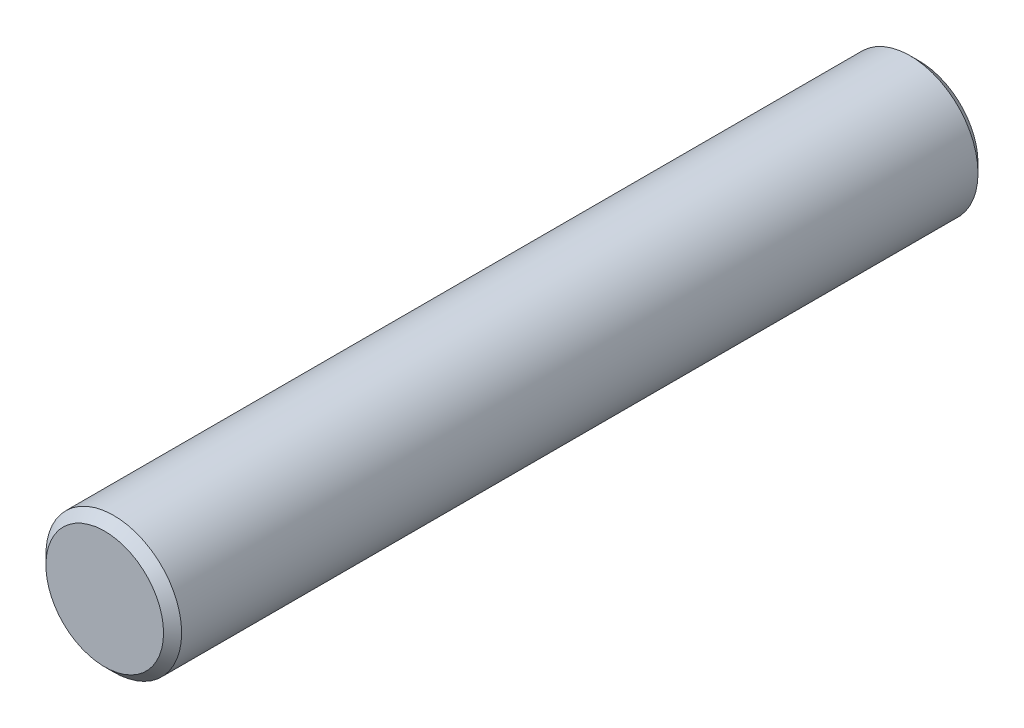
from build123d import *

# Parameters (mm, degrees)
PIN_PROFILE_3_R          = 1.5
PIN_BODY_3X18_DEPTH      = 9
END_CHAMFERS_0_2X45_SIZE = 0.2


with BuildPart() as part:
    # Pin Profile Ø3 → Pin Body Ø3x18 (new, symmetric)
    with BuildSketch(Plane.XY):
        Circle(PIN_PROFILE_3_R)
    extrude(amount=PIN_BODY_3X18_DEPTH, both=True)

    # End Chamfers 0.2x45°
    end_chamfers_0_2x45_edges = [part.edges().sort_by_distance(p)[0] for p in [
        (-1.5, 0, -9),
        (-1.5, 0, 9),
    ]]
    chamfer(end_chamfers_0_2x45_edges, length=END_CHAMFERS_0_2X45_SIZE)


solid = part.part
